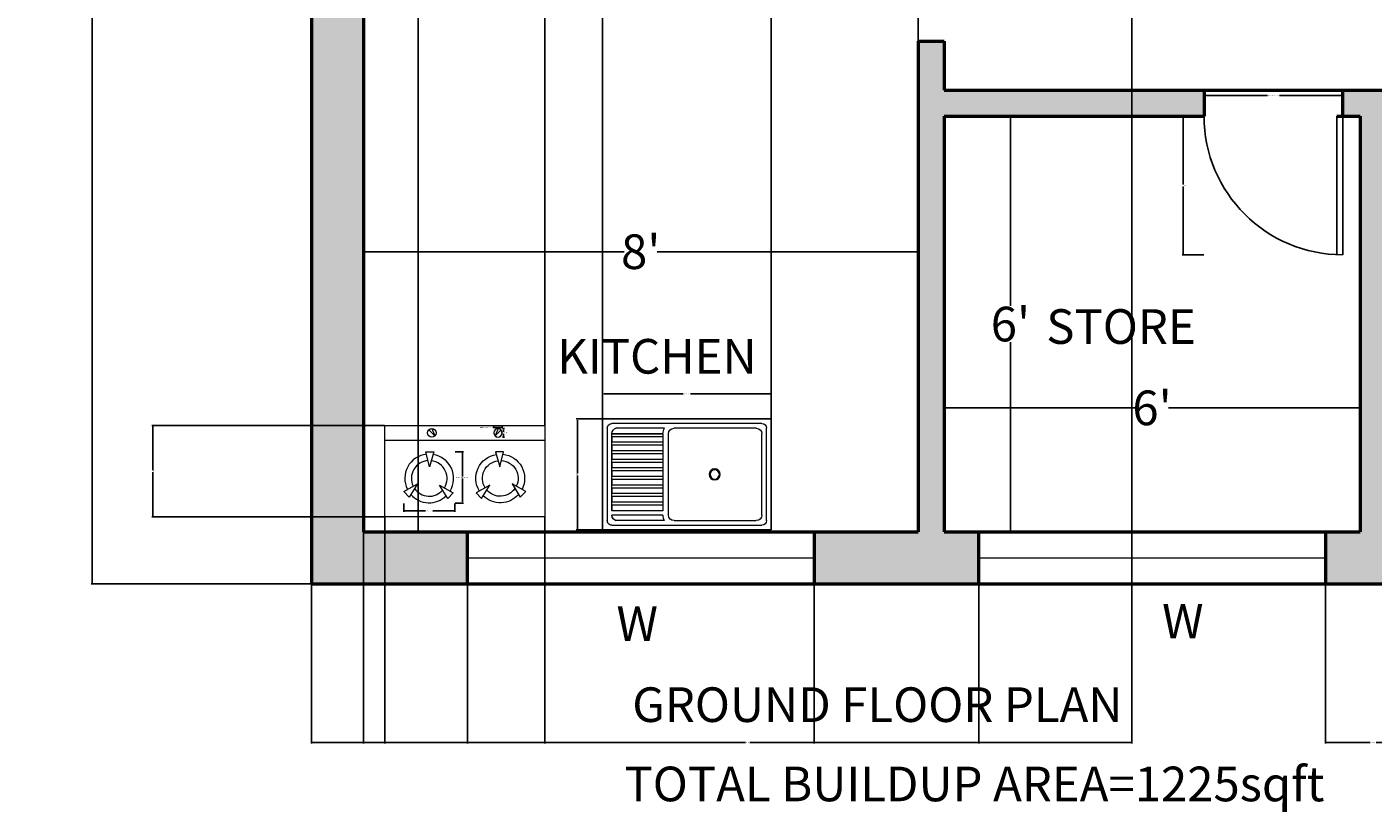
# Model space of a CAD drawing. Units: inches. Extents: x -22 to 470, y -437 to 97.
# Tile 1 of 9: x -22 to 211, y -437 to -301. Entities that reach past the tile are written whole.
import ezdxf

# ---------------------------------------------------------------- set-up
doc = ezdxf.new("R2010")
doc.units = ezdxf.units.IN
doc.header["$MEASUREMENT"] = 0
for name, color, linetype, lineweight in [('A-ANNO-DIMS', 2, 'Continuous', 18), ('A-ANNO-TEXT', 7, 'Continuous', 18), ('A-AREA-IDEN', 7, 'Continuous', 25), ('A-DOOR', 4, 'Continuous', 25), ('A-EQPM', 9, 'Continuous', 18), ('A-FLOR-FIXT', 9, 'Continuous', 20), ('A-GLAZ', 4, 'Continuous', 18), ('A-WALL', 7, 'Continuous', 50), ('A-WALL-PATT', 8, 'Continuous', 13)]:
    doc.layers.add(name, color=color, linetype=linetype, lineweight=lineweight)
doc.styles.get("Standard").update_dxf_attribs({"font": 'arial.ttf'})
doc.dimstyles.get("Standard").update_dxf_attribs({"dimtxt": 0.18, "dimasz": 0.18, "dimexe": 0.18, "dimexo": 0.0625, "dimgap": 0.09, "dimtad": 0, "dimtih": 1, "dimtoh": 1, "dimdec": 0, "dimzin": 0, "dimdsep": 46, "dimlunit": 3, "dimtxsty": 'Standard', "dimcen": 0.09, "dimadec": 0, "dimazin": 0, "dimtfac": 1, "dimtdec": 0, "dimtofl": 0, "dimtmove": 0, "dimatfit": 3, "dimfxl": 1, "dimtolj": 1, "dimtzin": 0, "dimarcsym": 0})

# ---------------------------------------------------------------- blocks, each defined once
blk = doc.blocks.new('М12 540х820')
for p, q in [((0, 540), (-820, 540)), ((-820, 540), (-820, 0)), ((0, 0), (0, 540)), ((-797.5, 495), (-797.5, 45)), ((-45, 517.5), (-775, 517.5)), ((-775, 468), (-775, 72)), ((-347.5, 495), (-748, 495)), ((-320.5, 468), (-320.5, 72)), ((-301.7, 495), (-64.8, 495)), ((-293.7, 468), (-293.7, 472.5)), ((-293.7, 468), (-45, 468)), ((-45, 469.5), (-45, 468)), ((-22.5, 45), (-22.5, 495)), ((-293.7, 446.6), (-45, 446.6)), ((-293.7, 419.6), (-293.7, 446.6)), ((-293.7, 419.6), (-45, 419.6)), ((-293.7, 405), (-45, 405)), ((-293.7, 378), (-293.7, 405)), ((-45, 419.6), (-45, 446.6)), ((-45, 378), (-45, 405)), ((-293.7, 378), (-45, 378)), ((-293.7, 336.4), (-293.7, 363.4)), ((-293.7, 363.4), (-45, 363.4)), ((-293.7, 336.4), (-45, 336.4)), ((-45, 336.4), (-45, 363.4)), ((-293.7, 294.7), (-293.7, 321.7)), ((-293.7, 321.7), (-45, 321.7)), ((-293.7, 294.7), (-45, 294.7)), ((-293.7, 253.1), (-293.7, 280.1)), ((-293.7, 280.1), (-45, 280.1)), ((-45, 294.7), (-45, 321.7)), ((-45, 253.1), (-45, 280.1)), ((-293.7, 253.1), (-45, 253.1)), ((-293.7, 211.5), (-293.7, 238.5)), ((-293.7, 238.5), (-45, 238.5)), ((-293.7, 211.5), (-45, 211.5)), ((-293.7, 169.9), (-293.7, 196.9)), ((-293.7, 196.9), (-45, 196.9)), ((-45, 211.5), (-45, 238.5)), ((-45, 169.9), (-45, 196.9)), ((-293.7, 169.9), (-45, 169.9)), ((-293.7, 128.2), (-293.7, 155.2)), ((-293.7, 155.2), (-45, 155.2)), ((-45, 128.2), (-45, 155.2)), ((-293.7, 128.2), (-45, 128.2)), ((-293.7, 113.6), (-45, 113.6)), ((-293.7, 86.6), (-293.7, 113.6)), ((-293.7, 86.6), (-45, 86.6)), ((-293.7, 72), (-45, 72)), ((-45, 86.6), (-45, 113.6)), ((-45, 70.5), (-45, 72)), ((-820, 0), (0, 0)), ((-775, 22.5), (-45, 22.5)), ((-748, 45), (-347.5, 45)), ((-301.7, 45), (-64.8, 45))]:
    blk.add_line(p, q)
at = {"ltscale": 0.06}
for p, q in [((-820, 0), (-820, 540)), ((-820, 540), (0, 540)), ((0, 540), (0, 536.9)), ((0, 536.9), (0, 0)), ((-293.7, 446.6), (-45, 446.6)), ((-293.7, 405), (-293.7, 446.6)), ((-293.7, 363.4), (-293.7, 405)), ((-45, 446.6), (-45, 419.6)), ((-45, 419.6), (-45, 378)), ((-293.7, 321.7), (-293.7, 363.4)), ((-45, 378), (-45, 336.4)), ((-45, 336.4), (-45, 294.7)), ((-293.7, 280.1), (-293.7, 321.7)), ((-293.7, 238.5), (-293.7, 280.1)), ((-45, 294.7), (-45, 253.1)), ((-293.7, 196.9), (-293.7, 238.5)), ((-293.7, 155.2), (-293.7, 196.9)), ((-45, 253.1), (-45, 211.5)), ((-45, 211.5), (-45, 169.9)), ((-293.7, 113.6), (-293.7, 155.2)), ((-45, 169.9), (-45, 128.2)), ((-293.7, 72), (-293.7, 113.6)), ((-45, 72), (-293.7, 72)), ((-45, 128.2), (-45, 86.6)), ((-45, 86.6), (-45, 72)), ((0, 0), (-820, 0))]:
    blk.add_line(p, q, dxfattribs=at)
at = {"extrusion": (0, 0, -1)}
for centre, major_axis, start_param, end_param in [((-775, 495), (-15.9, 15.9), -0.785398, 0.785398), ((-775, 495), (-15.9, 15.9), -0.785398, 0.785398), ((-748, 468), (-19.1, -19.1), 0.785398, 2.356194), ((-748, 468), (-19.1, -19.1), 0.785398, 2.356194), ((-347.5, 468), (-19.1, 19.1), 0.785398, 2.356194), ((-347.5, 468), (-19.1, 19.1), 0.785398, 2.356194), ((-343.2, 468), (-35, 35), 1.779263, 2.356194), ((-343.2, 468), (-35, 35), 1.779263, 2.356192), ((-343.2, 468), (-35, 35), 2.356192, 2.356194), ((-72.3, 468.8), (-19.3, 19.3), 1.0328, 2.38382), ((-72.3, 468.8), (-19.3, 19.3), 1.0328, 1.064673), ((-72.3, 468.8), (-19.3, 19.3), 1.064673, 2.328569), ((-45, 495), (-15.9, -15.9), 2.356194, 3.926991), ((-45, 495), (-15.9, -15.9), 2.356194, 3.926991), ((-72.3, 468.8), (-19.3, 19.3), 2.328569, 2.38382), ((-545.5, 270), (-19.1, -19.1), 3.926991, 10.210176), ((-545.5, 270), (-19.1, -19.1), 3.926991, 10.210176), ((-545.5, 270), (-15.9, -15.9), 3.926991, 10.210176), ((-545.5, 270), (-15.9, -15.9), 3.926991, 10.210176), ((-748, 72), (-19.1, 19.1), 3.926991, 5.497787), ((-748, 72), (-19.1, 19.1), 3.926991, 5.497787), ((-347.5, 72), (-19.1, -19.1), 3.926991, 5.497787), ((-347.5, 72), (-19.1, -19.1), 3.926991, 5.497787), ((-343.2, 72), (-35, -35), 3.926991, 4.503922), ((-343.2, 72), (-35, -35), 3.926991, 4.503922), ((-72.3, 71.2), (-19.3, -19.3), 3.899365, 5.250385), ((-72.3, 71.2), (-19.3, -19.3), 3.954617, 5.218512), ((-72.3, 71.2), (-19.3, -19.3), 3.899365, 3.954617), ((-775, 45), (-15.9, -15.9), 5.497787, 7.068583), ((-775, 45), (-15.9, -15.9), 5.497787, 7.068583), ((-72.3, 71.2), (-19.3, -19.3), 5.218512, 5.250385), ((-45, 45), (-15.9, 15.9), 2.356194, 3.926991), ((-45, 45), (-15.9, 15.9), 2.356194, 3.926991)]:
    blk.add_ellipse(centre, major_axis=major_axis, ratio=1, start_param=start_param, end_param=end_param, dxfattribs=at)
blk = doc.blocks.new('*D3')
at = {"layer": 'A-ANNO-DIMS', "color": 0, "lineweight": -2, "transparency": 16777216}
for p, q in [((26.86, 13.24), (-11.18, 13.24)), ((-11, 13.06), (-11, -189.1)), ((-11, -397.58), (-11, -195.41)), ((26.86, -397.76), (-11.18, -397.76))]:
    blk.add_line(p, q, dxfattribs=at)
at = {"layer": 'A-ANNO-DIMS', "color": 0, "transparency": 16777216}
for points in [[(-11.03, 13.06), (-10.97, 13.06), (-11, 13.24)], [(-11.03, -397.58), (-10.97, -397.58), (-11, -397.76)]]:
    blk.add_solid(points, dxfattribs=at)
at = {"layer": 'Defpoints', "color": 0, "transparency": 16777216}
for p in [(26.92, 13.24), (-11, -397.76), (26.92, -397.76)]:
    blk.add_point(p, dxfattribs=at)
at = {"layer": 'A-ANNO-DIMS', "color": 0, "transparency": 16777216, "insert": (-11, -192.26), "char_height": 6, "attachment_point": 5}
blk.add_mtext('\\A1;34\'-3"', dxfattribs=at)
blk = doc.blocks.new('*D15')
at = {"layer": 'A-ANNO-DIMS', "color": 0, "lineweight": -2, "transparency": 16777216}
for p, q in [((35.92, -346.19), (35.92, -340.05)), ((131.92, -346.19), (131.92, -340.05)), ((36.1, -340.23), (81.07, -340.23)), ((131.74, -340.23), (86.78, -340.23))]:
    blk.add_line(p, q, dxfattribs=at)
at = {"layer": 'A-ANNO-DIMS', "color": 0, "transparency": 16777216}
for points in [[(36.1, -340.2), (36.1, -340.26), (35.92, -340.23)], [(131.74, -340.2), (131.74, -340.26), (131.92, -340.23)]]:
    blk.add_solid(points, dxfattribs=at)
at = {"layer": 'Defpoints', "color": 0, "transparency": 16777216}
for p in [(35.92, -340.23), (35.92, -346.25), (131.92, -346.25)]:
    blk.add_point(p, dxfattribs=at)
at = {"layer": 'A-ANNO-DIMS', "color": 0, "transparency": 16777216, "insert": (83.92, -340.23), "char_height": 6, "attachment_point": 5}
blk.add_mtext("\\A1;8'", dxfattribs=at)
blk = doc.blocks.new('*D16')
at = {"layer": 'A-ANNO-DIMS', "color": 0, "lineweight": -2, "transparency": 16777216}
for p, q in [((136.42, -367.21), (136.42, -367.09)), ((136.6, -367.27), (169.55, -367.27)), ((208.24, -367.27), (175.29, -367.27)), ((208.42, -367.21), (208.42, -367.09))]:
    blk.add_line(p, q, dxfattribs=at)
at = {"layer": 'A-ANNO-DIMS', "color": 0, "transparency": 16777216}
for points in [[(136.6, -367.24), (136.6, -367.3), (136.42, -367.27)], [(208.24, -367.24), (208.24, -367.3), (208.42, -367.27)]]:
    blk.add_solid(points, dxfattribs=at)
at = {"layer": 'Defpoints', "color": 0, "transparency": 16777216}
for p in [(136.42, -367.27), (136.42, -367.27), (208.42, -367.27)]:
    blk.add_point(p, dxfattribs=at)
at = {"layer": 'A-ANNO-DIMS', "color": 0, "transparency": 16777216, "insert": (172.42, -367.27), "char_height": 6, "attachment_point": 5}
blk.add_mtext("\\A1;6'", dxfattribs=at)
blk = doc.blocks.new('*D17')
at = {"layer": 'A-ANNO-DIMS', "color": 0, "lineweight": -2, "transparency": 16777216}
for p, q in [((148.79, -316.76), (147.73, -316.76)), ((147.91, -316.94), (147.91, -349.6)), ((147.91, -388.58), (147.91, -355.91)), ((148.79, -388.76), (147.73, -388.76))]:
    blk.add_line(p, q, dxfattribs=at)
at = {"layer": 'A-ANNO-DIMS', "color": 0, "transparency": 16777216}
for points in [[(147.88, -316.94), (147.94, -316.94), (147.91, -316.76)], [(147.88, -388.58), (147.94, -388.58), (147.91, -388.76)]]:
    blk.add_solid(points, dxfattribs=at)
at = {"layer": 'Defpoints', "color": 0, "transparency": 16777216}
for p in [(148.85, -316.76), (147.91, -388.76), (148.85, -388.76)]:
    blk.add_point(p, dxfattribs=at)
at = {"layer": 'A-ANNO-DIMS', "color": 0, "transparency": 16777216, "insert": (147.91, -352.76), "char_height": 6, "attachment_point": 5}
blk.add_mtext("\\A1;6'", dxfattribs=at)
blk = doc.blocks.new('*D20')
at = {"layer": 'A-ANNO-DIMS', "color": 0, "lineweight": -2, "transparency": 16777216}
for p, q in [((45.66, -196.76), (45.23, -196.76)), ((45.41, -196.94), (45.41, -289.6)), ((45.41, -388.58), (45.41, -295.91)), ((45.66, -388.76), (45.23, -388.76))]:
    blk.add_line(p, q, dxfattribs=at)
at = {"layer": 'A-ANNO-DIMS', "color": 0, "transparency": 16777216}
for points in [[(45.38, -196.94), (45.44, -196.94), (45.41, -196.76)], [(45.38, -388.58), (45.44, -388.58), (45.41, -388.76)]]:
    blk.add_solid(points, dxfattribs=at)
at = {"layer": 'Defpoints', "color": 0, "transparency": 16777216}
for p in [(45.73, -196.76), (45.41, -388.76), (45.73, -388.76)]:
    blk.add_point(p, dxfattribs=at)
at = {"layer": 'A-ANNO-DIMS', "color": 0, "transparency": 16777216, "insert": (45.41, -292.76), "char_height": 6, "attachment_point": 5}
blk.add_mtext("\\A1;16'", dxfattribs=at)
blk = doc.blocks.new('DOOR-SWING-24')
for p, q in [((23, 24), (23, 0)), ((24, 24), (24, 0))]:
    blk.add_line(p, q)
blk.add_arc((24, 24), 24, 180, 270)
blk = doc.blocks.new('COOKTOP-BURNER')
for p, q in [((4.49, 6.22), (3.84, 8.82)), ((3.84, 8.82), (5.21, 8.82)), ((5.21, 8.82), (4.49, 6.22)), ((0, 1.96), (2.36, 3.28)), ((2.36, 3.28), (0.96, 0.99)), ((7.64, 0.74), (6.21, 3.03)), ((6.21, 3.03), (8.57, 1.74)), ((0.96, 0.99), (0, 1.96)), ((8.57, 1.74), (7.64, 0.74))]:
    blk.add_line(p, q)
for radius, start, end in [(4.22, 96.4005, 206.769), (3.09, 93.5753, 205.9207), (3.09, 327.9778, 83.02), (4.22, 328.853, 80.7562), (3.09, 214.5561, 318.8027), (4.22, 221.2225, 314.1627)]:
    blk.add_arc((4.41, 4.22), radius, start, end)
blk = doc.blocks.new('COOKTOP-DIAL')
at = {"ltscale": 20}
for p, q in [((1.25, 0.22), (0.21, 1.24)), ((0.73, 1.46), (1.25, 0.22))]:
    blk.add_line(p, q, dxfattribs=at)
blk.add_circle((0.73, 0.73), 0.728, dxfattribs=at)
blk = doc.blocks.new('WINDOW-60-SASH')
for p, q in [((0, 9), (60, 9)), ((0, 4.5), (60, 4.5)), ((60, 0), (0, 0))]:
    blk.add_line(p, q)
blk = doc.blocks.new('*D37')
at = {"layer": 'A-ANNO-DIMS', "color": 0, "lineweight": -2, "transparency": 16777216}
for p, q in [((181.42, -316.69), (181.42, -312.98)), ((181.6, -313.16), (192.38, -313.16)), ((205.24, -313.16), (194.47, -313.16)), ((205.42, -316.69), (205.42, -312.98))]:
    blk.add_line(p, q, dxfattribs=at)
at = {"layer": 'A-ANNO-DIMS', "color": 0, "transparency": 16777216}
for points in [[(181.6, -313.13), (181.6, -313.19), (181.42, -313.16)], [(205.24, -313.13), (205.24, -313.19), (205.42, -313.16)]]:
    blk.add_solid(points, dxfattribs=at)
at = {"layer": 'Defpoints', "color": 0, "transparency": 16777216}
for p in [(205.42, -313.16), (181.42, -316.76), (205.42, -316.76)]:
    blk.add_point(p, dxfattribs=at)
at = {"layer": 'A-ANNO-DIMS', "color": 0, "transparency": 16777216, "insert": (193.42, -313.16), "char_height": 0.18, "attachment_point": 5}
blk.add_mtext('\\A1;DOOR 2\'-0" TYP.', dxfattribs=at)
blk = doc.blocks.new('*D38')
at = {"layer": 'A-ANNO-DIMS', "color": 0, "lineweight": -2, "transparency": 16777216}
for p, q in [((181.36, -316.76), (177.64, -316.76)), ((177.82, -316.94), (177.82, -328.57)), ((177.82, -340.58), (177.82, -328.94)), ((181.36, -340.76), (177.64, -340.76))]:
    blk.add_line(p, q, dxfattribs=at)
at = {"layer": 'A-ANNO-DIMS', "color": 0, "transparency": 16777216}
for points in [[(177.79, -316.94), (177.85, -316.94), (177.82, -316.76)], [(177.79, -340.58), (177.85, -340.58), (177.82, -340.76)]]:
    blk.add_solid(points, dxfattribs=at)
at = {"layer": 'Defpoints', "color": 0, "transparency": 16777216}
for p in [(177.82, -316.76), (181.42, -316.76), (181.42, -340.76)]:
    blk.add_point(p, dxfattribs=at)
at = {"layer": 'A-ANNO-DIMS', "color": 0, "transparency": 16777216, "insert": (177.82, -328.76), "char_height": 0.18, "attachment_point": 5}
blk.add_mtext('\\A1;2\'-0" TYP.', dxfattribs=at)
blk = doc.blocks.new('*D55')
at = {"layer": 'A-ANNO-DIMS', "color": 0, "lineweight": -2, "transparency": 16777216}
for p, q in [((58.49, -370.65), (58.31, -370.65)), ((58.49, -370.81), (58.49, -370.47)), ((59.77, -370.65), (58.67, -370.65)), ((59.95, -370.81), (59.95, -370.47))]:
    blk.add_line(p, q, dxfattribs=at)
at = {"layer": 'A-ANNO-DIMS', "color": 0, "transparency": 16777216}
for points in [[(58.67, -370.62), (58.67, -370.68), (58.49, -370.65)], [(59.77, -370.62), (59.77, -370.68), (59.95, -370.65)]]:
    blk.add_solid(points, dxfattribs=at)
at = {"layer": 'Defpoints', "color": 0, "transparency": 16777216}
for p in [(58.49, -370.65), (58.49, -370.87), (59.95, -370.87)]:
    blk.add_point(p, dxfattribs=at)
at = {"layer": 'A-ANNO-DIMS', "color": 0, "transparency": 16777216, "insert": (57.15, -370.65), "char_height": 0.18, "attachment_point": 5}
blk.add_mtext('\\A1;DIAL 0\'-1 1/2" TYP.', dxfattribs=at)
blk = doc.blocks.new('*D56')
at = {"layer": 'A-ANNO-DIMS', "color": 0, "lineweight": -2, "transparency": 16777216}
for p, q in [((60.01, -370.87), (60.35, -370.87)), ((60.01, -372.33), (60.35, -372.33)), ((60.17, -371.05), (60.17, -371.42)), ((60.17, -372.15), (60.17, -371.78))]:
    blk.add_line(p, q, dxfattribs=at)
at = {"layer": 'A-ANNO-DIMS', "color": 0, "transparency": 16777216}
for points in [[(60.14, -371.05), (60.2, -371.05), (60.17, -370.87)], [(60.14, -372.15), (60.2, -372.15), (60.17, -372.33)]]:
    blk.add_solid(points, dxfattribs=at)
at = {"layer": 'Defpoints', "color": 0, "transparency": 16777216}
for p in [(59.95, -370.87), (59.95, -372.33), (60.17, -370.87)]:
    blk.add_point(p, dxfattribs=at)
at = {"layer": 'A-ANNO-DIMS', "color": 0, "transparency": 16777216, "insert": (60.17, -371.6), "char_height": 0.18, "attachment_point": 5}
blk.add_mtext('\\A1;0\'-1 1/2" TYP.', dxfattribs=at)
blk = doc.blocks.new('*D57')
at = {"layer": 'A-ANNO-DIMS', "color": 0, "lineweight": -2, "transparency": 16777216}
for p, q in [((51.8, -374.88), (53.24, -374.88)), ((53.06, -375.06), (53.06, -379.13)), ((53.06, -383.57), (53.06, -379.5)), ((51.8, -383.75), (53.24, -383.75))]:
    blk.add_line(p, q, dxfattribs=at)
at = {"layer": 'A-ANNO-DIMS', "color": 0, "transparency": 16777216}
for points in [[(53.03, -375.06), (53.09, -375.06), (53.06, -374.88)], [(53.03, -383.57), (53.09, -383.57), (53.06, -383.75)]]:
    blk.add_solid(points, dxfattribs=at)
at = {"layer": 'Defpoints', "color": 0, "transparency": 16777216}
for p in [(51.73, -374.88), (53.06, -374.88), (51.73, -383.75)]:
    blk.add_point(p, dxfattribs=at)
at = {"layer": 'A-ANNO-DIMS', "color": 0, "transparency": 16777216, "insert": (53.06, -379.32), "char_height": 0.18, "attachment_point": 5}
blk.add_mtext('\\A1;BURNER 0\'-9" TYP.', dxfattribs=at)
blk = doc.blocks.new('*D58')
at = {"layer": 'A-ANNO-DIMS', "color": 0, "lineweight": -2, "transparency": 16777216}
for p, q in [((42.9, -383.81), (42.9, -385.26)), ((51.73, -383.81), (51.73, -385.26)), ((43.08, -385.08), (46.68, -385.08)), ((51.55, -385.08), (47.96, -385.08))]:
    blk.add_line(p, q, dxfattribs=at)
at = {"layer": 'A-ANNO-DIMS', "color": 0, "transparency": 16777216}
for points in [[(43.08, -385.05), (43.08, -385.11), (42.9, -385.08)], [(51.55, -385.05), (51.55, -385.11), (51.73, -385.08)]]:
    blk.add_solid(points, dxfattribs=at)
at = {"layer": 'Defpoints', "color": 0, "transparency": 16777216}
for p in [(42.9, -383.75), (51.73, -383.75), (51.73, -385.08)]:
    blk.add_point(p, dxfattribs=at)
at = {"layer": 'A-ANNO-DIMS', "color": 0, "transparency": 16777216, "insert": (47.32, -385.08), "char_height": 0.18, "attachment_point": 5}
blk.add_mtext('\\A1;0\'-9" TYP.', dxfattribs=at)
blk = doc.blocks.new('*D59')
at = {"layer": 'A-ANNO-DIMS', "color": 0, "lineweight": -2, "transparency": 16777216}
for p, q in [((77.33, -369.14), (77.33, -364.65)), ((77.51, -364.83), (91.25, -364.83)), ((106.3, -364.83), (92.56, -364.83)), ((106.48, -369.14), (106.48, -364.65))]:
    blk.add_line(p, q, dxfattribs=at)
at = {"layer": 'A-ANNO-DIMS', "color": 0, "transparency": 16777216}
for points in [[(77.51, -364.8), (77.51, -364.86), (77.33, -364.83)], [(106.3, -364.8), (106.3, -364.86), (106.48, -364.83)]]:
    blk.add_solid(points, dxfattribs=at)
at = {"layer": 'Defpoints', "color": 0, "transparency": 16777216}
for p in [(77.33, -364.83), (77.33, -369.2), (106.48, -369.2)]:
    blk.add_point(p, dxfattribs=at)
at = {"layer": 'A-ANNO-DIMS', "color": 0, "transparency": 16777216, "insert": (91.91, -364.83), "char_height": 0.18, "attachment_point": 5}
blk.add_mtext('\\A1;SINK 2\'-5"', dxfattribs=at)
blk = doc.blocks.new('*D60')
at = {"layer": 'A-ANNO-DIMS', "color": 0, "lineweight": -2, "transparency": 16777216}
for p, q in [((77.27, -369.2), (72.77, -369.2)), ((72.95, -369.38), (72.95, -378.62)), ((72.95, -388.22), (72.95, -378.98)), ((77.27, -388.4), (72.77, -388.4))]:
    blk.add_line(p, q, dxfattribs=at)
at = {"layer": 'A-ANNO-DIMS', "color": 0, "transparency": 16777216}
for points in [[(72.92, -369.38), (72.98, -369.38), (72.95, -369.2)], [(72.92, -388.22), (72.98, -388.22), (72.95, -388.4)]]:
    blk.add_solid(points, dxfattribs=at)
at = {"layer": 'Defpoints', "color": 0, "transparency": 16777216}
for p in [(77.33, -369.2), (72.95, -388.4), (77.33, -388.4)]:
    blk.add_point(p, dxfattribs=at)
at = {"layer": 'A-ANNO-DIMS', "color": 0, "transparency": 16777216, "insert": (72.95, -378.8), "char_height": 0.18, "attachment_point": 5}
blk.add_mtext('\\A1;1\'-7"', dxfattribs=at)
blk = doc.blocks.new('*D62')
at = {"layer": 'A-ANNO-DIMS', "color": 0, "lineweight": -2, "transparency": 16777216}
for p, q in [((35.92, -192.32), (35.92, -425.39)), ((168.92, -192.32), (168.92, -425.39)), ((36.1, -425.21), (102.03, -425.21)), ((168.74, -425.21), (102.81, -425.21))]:
    blk.add_line(p, q, dxfattribs=at)
at = {"layer": 'A-ANNO-DIMS', "color": 0, "transparency": 16777216}
for points in [[(36.1, -425.18), (36.1, -425.24), (35.92, -425.21)], [(168.74, -425.18), (168.74, -425.24), (168.92, -425.21)]]:
    blk.add_solid(points, dxfattribs=at)
at = {"layer": 'Defpoints', "color": 0, "transparency": 16777216}
for p in [(35.92, -192.26), (168.92, -192.26), (168.92, -425.21)]:
    blk.add_point(p, dxfattribs=at)
at = {"layer": 'A-ANNO-DIMS', "color": 0, "transparency": 16777216, "insert": (102.42, -425.21), "char_height": 0.18, "attachment_point": 5}
blk.add_mtext('\\A1;11\'-1"', dxfattribs=at)
blk = doc.blocks.new('*D72')
at = {"layer": 'A-ANNO-DIMS', "color": 0, "lineweight": -2, "transparency": 16777216}
for p, q in [((26.92, -397.82), (26.92, -425.39)), ((53.92, -397.82), (53.92, -425.39)), ((27.1, -425.21), (40.09, -425.21)), ((53.74, -425.21), (40.75, -425.21))]:
    blk.add_line(p, q, dxfattribs=at)
at = {"layer": 'A-ANNO-DIMS', "color": 0, "transparency": 16777216}
for points in [[(27.1, -425.18), (27.1, -425.24), (26.92, -425.21)], [(53.74, -425.18), (53.74, -425.24), (53.92, -425.21)]]:
    blk.add_solid(points, dxfattribs=at)
at = {"layer": 'Defpoints', "color": 0, "transparency": 16777216}
for p in [(26.92, -397.76), (53.92, -397.76), (53.92, -425.21)]:
    blk.add_point(p, dxfattribs=at)
at = {"layer": 'A-ANNO-DIMS', "color": 0, "transparency": 16777216, "insert": (40.42, -425.21), "char_height": 0.18, "attachment_point": 5}
blk.add_mtext('\\A1;2\'-3"', dxfattribs=at)
blk = doc.blocks.new('*D73')
at = {"layer": 'A-ANNO-DIMS', "color": 0, "lineweight": -2, "transparency": 16777216}
for p, q in [((113.92, -397.82), (113.92, -425.39)), ((142.42, -397.82), (142.42, -425.39)), ((114.1, -425.21), (127.63, -425.21)), ((142.24, -425.21), (128.71, -425.21))]:
    blk.add_line(p, q, dxfattribs=at)
at = {"layer": 'A-ANNO-DIMS', "color": 0, "transparency": 16777216}
for points in [[(114.1, -425.18), (114.1, -425.24), (113.92, -425.21)], [(142.24, -425.18), (142.24, -425.24), (142.42, -425.21)]]:
    blk.add_solid(points, dxfattribs=at)
at = {"layer": 'Defpoints', "color": 0, "transparency": 16777216}
for p in [(113.92, -397.76), (142.42, -397.76), (142.42, -425.21)]:
    blk.add_point(p, dxfattribs=at)
at = {"layer": 'A-ANNO-DIMS', "color": 0, "transparency": 16777216, "insert": (128.17, -425.21), "char_height": 0.18, "attachment_point": 5}
blk.add_mtext('\\A1;2\'-4 1/2"', dxfattribs=at)
blk = doc.blocks.new('*D74')
at = {"layer": 'A-ANNO-DIMS', "color": 0, "lineweight": -2, "transparency": 16777216}
for p, q in [((202.42, -397.82), (202.42, -425.39)), ((218.92, -397.82), (218.92, -425.39)), ((202.6, -425.21), (210.14, -425.21)), ((218.74, -425.21), (211.2, -425.21))]:
    blk.add_line(p, q, dxfattribs=at)
at = {"layer": 'A-ANNO-DIMS', "color": 0, "transparency": 16777216}
for points in [[(202.6, -425.18), (202.6, -425.24), (202.42, -425.21)], [(218.74, -425.18), (218.74, -425.24), (218.92, -425.21)]]:
    blk.add_solid(points, dxfattribs=at)
at = {"layer": 'Defpoints', "color": 0, "transparency": 16777216}
for p in [(202.42, -397.76), (218.92, -397.76), (218.92, -425.21)]:
    blk.add_point(p, dxfattribs=at)
at = {"layer": 'A-ANNO-DIMS', "color": 0, "transparency": 16777216, "insert": (210.67, -425.21), "char_height": 0.18, "attachment_point": 5}
blk.add_mtext('\\A1;1\'-4 1/2"', dxfattribs=at)
blk = doc.blocks.new('*D81')
at = {"layer": 'A-ANNO-DIMS', "color": 0, "lineweight": -2, "transparency": 16777216}
for p, q in [((39.64, -386.21), (39.64, -425.39)), ((67.35, -386.21), (67.35, -425.39)), ((39.82, -425.21), (52.95, -425.21)), ((67.17, -425.21), (54.04, -425.21))]:
    blk.add_line(p, q, dxfattribs=at)
at = {"layer": 'A-ANNO-DIMS', "color": 0, "transparency": 16777216}
for points in [[(39.82, -425.18), (39.82, -425.24), (39.64, -425.21)], [(67.17, -425.18), (67.17, -425.24), (67.35, -425.21)]]:
    blk.add_solid(points, dxfattribs=at)
at = {"layer": 'Defpoints', "color": 0, "transparency": 16777216}
for p in [(39.64, -386.15), (67.35, -386.15), (67.35, -425.21)]:
    blk.add_point(p, dxfattribs=at)
at = {"layer": 'A-ANNO-DIMS', "color": 0, "transparency": 16777216, "insert": (53.49, -425.21), "char_height": 0.18, "attachment_point": 5}
blk.add_mtext('\\A1;2\'-3 1/2"', dxfattribs=at)
blk = doc.blocks.new('*D82')
at = {"layer": 'A-ANNO-DIMS', "color": 0, "lineweight": -2, "transparency": 16777216}
for p, q in [((39.58, -370.32), (-0.71, -370.32)), ((-0.53, -370.5), (-0.53, -378.05)), ((-0.53, -385.97), (-0.53, -378.41)), ((39.58, -386.15), (-0.71, -386.15))]:
    blk.add_line(p, q, dxfattribs=at)
at = {"layer": 'A-ANNO-DIMS', "color": 0, "transparency": 16777216}
for points in [[(-0.56, -370.5), (-0.5, -370.5), (-0.53, -370.32)], [(-0.56, -385.97), (-0.5, -385.97), (-0.53, -386.15)]]:
    blk.add_solid(points, dxfattribs=at)
at = {"layer": 'Defpoints', "color": 0, "transparency": 16777216}
for p in [(39.64, -370.32), (-0.53, -386.15), (39.64, -386.15)]:
    blk.add_point(p, dxfattribs=at)
at = {"layer": 'A-ANNO-DIMS', "color": 0, "transparency": 16777216, "insert": (-0.53, -378.23), "char_height": 0.18, "attachment_point": 5}
blk.add_mtext('\\A1;1\'-4"', dxfattribs=at)
blk = doc.blocks.new('*D83')
at = {"layer": 'A-ANNO-DIMS', "color": 0, "lineweight": -2, "transparency": 16777216}
for p, q in [((67.35, -370.26), (67.35, 40.87)), ((67.53, 40.69), (71.94, 40.69)), ((77.15, 40.69), (72.74, 40.69)), ((77.33, -369.14), (77.33, 40.87))]:
    blk.add_line(p, q, dxfattribs=at)
at = {"layer": 'A-ANNO-DIMS', "color": 0, "transparency": 16777216}
for points in [[(67.53, 40.72), (67.53, 40.66), (67.35, 40.69)], [(77.15, 40.72), (77.15, 40.66), (77.33, 40.69)]]:
    blk.add_solid(points, dxfattribs=at)
at = {"layer": 'Defpoints', "color": 0, "transparency": 16777216}
for p in [(77.33, 40.69), (67.35, -370.32), (77.33, -369.2)]:
    blk.add_point(p, dxfattribs=at)
at = {"layer": 'A-ANNO-DIMS', "color": 0, "transparency": 16777216, "insert": (72.34, 40.69), "char_height": 0.18, "attachment_point": 5}
blk.add_mtext('\\A1;0\'-10"', dxfattribs=at)
blk = doc.blocks.new('*D84')
at = {"layer": 'A-ANNO-DIMS', "color": 0, "lineweight": -2, "transparency": 16777216}
for p, q in [((106.48, -369.14), (106.48, 40.87)), ((106.66, 40.69), (118.66, 40.69)), ((131.74, 40.69), (119.74, 40.69)), ((131.92, -388.69), (131.92, 40.87))]:
    blk.add_line(p, q, dxfattribs=at)
at = {"layer": 'A-ANNO-DIMS', "color": 0, "transparency": 16777216}
for points in [[(106.66, 40.72), (106.66, 40.66), (106.48, 40.69)], [(131.74, 40.72), (131.74, 40.66), (131.92, 40.69)]]:
    blk.add_solid(points, dxfattribs=at)
at = {"layer": 'Defpoints', "color": 0, "transparency": 16777216}
for p in [(131.92, 40.69), (106.48, -369.2), (131.92, -388.76)]:
    blk.add_point(p, dxfattribs=at)
at = {"layer": 'A-ANNO-DIMS', "color": 0, "transparency": 16777216, "insert": (119.2, 40.69), "char_height": 0.18, "attachment_point": 5}
blk.add_mtext('\\A1;2\'-1 1/2"', dxfattribs=at)

msp = doc.modelspace()

# ---------------------------------------------------------------- hatches: boundary and pattern name
at = {"layer": 'A-WALL-PATT'}
h = msp.add_hatch(color=256, dxfattribs=at)
h.dxf.hatch_style = 1
h.paths.add_polyline_path([(130.42, 13.24), (26.92, 13.24), (26.92, -43.76), (35.92, -43.76), (35.92, 4.24), (83.92, 4.24), (83.92, 1.24), (88.42, 1.24), (88.42, 4.24), (130.42, 4.24)])
h.paths.add_polyline_path([(266.92, 13.24), (190.42, 13.24), (190.42, 4.24), (232.42, 4.24), (232.42, -115.76), (229.42, -115.76), (229.42, -120.26), (239.92, -120.26), (239.92, -115.76), (236.92, -115.76), (236.92, 4.24), (266.92, 4.24)])
h.paths.add_polyline_path([(442.42, 13.24), (326.92, 13.24), (326.92, 4.24), (356.92, 4.24), (356.92, 1.24), (361.42, 1.24), (361.42, 4.24), (433.42, 4.24), (433.42, -49.38), (442.42, -49.38)])
h.paths.add_polyline_path([(442.42, -73.38), (433.42, -73.38), (433.42, -115.76), (361.42, -115.76), (361.42, -22.76), (356.92, -22.76), (356.92, -115.76), (263.92, -115.76), (263.92, -120.26), (332.92, -120.26), (332.92, -123.26), (337.42, -123.26), (337.42, -120.26), (433.42, -120.26), (433.42, -148.49), (442.42, -148.49)])
h.paths.add_polyline_path([(205.42, -115.76), (88.42, -115.76), (88.42, -22.76), (83.92, -22.76), (83.92, -115.76), (35.92, -115.76), (35.92, -67.76), (26.92, -67.76), (26.92, -126.26), (35.92, -126.26), (35.92, -120.26), (205.42, -120.26)])
h.paths.add_polyline_path([(35.92, -196.76), (168.92, -196.76), (168.92, -192.26), (35.92, -192.26), (35.92, -186.26), (26.92, -186.26), (26.92, -224.25), (35.92, -224.25)])
h.paths.add_polyline_path([(35.92, -284.25), (26.92, -284.25), (26.92, -397.76), (53.92, -397.76), (53.92, -388.76), (35.92, -388.76)])
h.paths.add_polyline_path([(142.42, -388.76), (136.42, -388.76), (136.42, -316.76), (181.42, -316.76), (181.42, -312.26), (136.42, -312.26), (136.42, -303.75), (131.92, -303.75), (131.92, -388.76), (113.92, -388.76), (113.92, -397.76), (142.42, -397.76)])
h.paths.add_polyline_path([(218.92, -388.76), (212.92, -388.76), (212.92, -312.26), (205.42, -312.26), (205.42, -316.76), (208.42, -316.76), (208.42, -388.76), (202.42, -388.76), (202.42, -397.76), (218.92, -397.76)])
h.paths.add_polyline_path([(306.75, -388.76), (289.42, -388.76), (289.42, -316.76), (284.92, -316.76), (284.92, -388.76), (278.92, -388.76), (278.92, -397.76), (306.75, -397.76)])
h.paths.add_polyline_path([(391.42, -388.76), (366.75, -388.76), (366.75, -397.76), (391.42, -397.76)], flags=17)
h.paths.add_polyline_path([(442.42, -172.49), (433.42, -172.49), (433.42, -192.26), (337.42, -192.26), (337.42, -147.26), (332.92, -147.26), (332.92, -196.76), (433.42, -196.76), (433.42, -388.76), (427.42, -388.76), (427.42, -397.76), (442.42, -397.76)])

# ---------------------------------------------------------------- linework, layer by layer
at = {"layer": 'A-EQPM'}
msp.add_line((39.64, -372.89), (67.35, -372.89), dxfattribs=at)
msp.add_lwpolyline([(67.35, -386.15), (39.64, -386.15), (39.64, -370.32), (67.35, -370.32)], close=True, dxfattribs=at)
at = {"layer": 'A-WALL'}
for p, q in [((26.92, 13.24), (26.92, -397.76)), ((35.92, -196.76), (35.92, -388.76)), ((131.92, -303.75), (131.92, -388.76)), ((131.92, -303.75), (136.42, -303.75)), ((136.42, -303.75), (136.42, -312.26)), ((136.42, -312.26), (212.92, -312.26)), ((181.42, -312.26), (181.42, -316.76)), ((205.42, -316.76), (205.42, -312.26)), ((136.42, -316.76), (181.42, -316.76)), ((136.42, -316.76), (136.42, -388.76)), ((204.42, -316.76), (208.42, -316.76)), ((208.42, -316.76), (208.42, -388.76)), ((35.92, -388.76), (131.92, -388.76)), ((53.92, -397.76), (53.92, -388.76)), ((113.92, -388.76), (113.92, -397.76)), ((136.42, -388.76), (208.42, -388.76)), ((142.42, -397.76), (142.42, -388.76)), ((202.42, -388.76), (202.42, -397.76)), ((26.92, -397.76), (391.42, -397.76))]:
    msp.add_line(p, q, dxfattribs=at)

# ---------------------------------------------------------------- block references
at = {"layer": 'A-DOOR'}
msp.add_blockref('DOOR-SWING-24', (181.42, -340.76), dxfattribs=at)
at = {"layer": 'A-EQPM'}
for name, p in [('COOKTOP-DIAL', (47.04, -372.33)), ('COOKTOP-BURNER', (42.9, -383.71))]:
    msp.add_blockref(name, p, dxfattribs=at)
at = {"layer": 'A-EQPM', "extrusion": (0, 0, -1), "zscale": -1}
for name, p in [('COOKTOP-DIAL', (-59.95, -372.33)), ('COOKTOP-BURNER', (-64.02, -383.71))]:
    msp.add_blockref(name, p, dxfattribs=at)
at = {"layer": 'A-FLOR-FIXT', "xscale": 0.0355567693074003, "yscale": 0.0355567693074003, "zscale": 0.0355567693074003, "rotation": 180}
msp.add_blockref('М12 540х820', (77.33, -369.2), dxfattribs=at)
at = {"layer": 'A-GLAZ'}
for p in [(53.92, -397.76), (142.42, -397.76)]:
    msp.add_blockref('WINDOW-60-SASH', p, dxfattribs=at)

# ---------------------------------------------------------------- texts
at = {"layer": 'A-ANNO-TEXT', "char_height": 6, "attachment_point": 1}
for s, insert in [('W', (79.72, -401.63)), ('W', (174.15, -401.21)), ('GROUND FLOOR PLAN', (82.45, -415.67)), ('TOTAL BUILDUP AREA=1225sqft', (81.1, -429.4))]:
    msp.add_mtext(s, dxfattribs=dict(at, insert=insert))
at = {"layer": 'A-AREA-IDEN', "char_height": 6, "attachment_point": 1}
for s, insert in [('STORE', (154.11, -350.19)), ('KITCHEN', (69.48, -355.34))]:
    msp.add_mtext(s, dxfattribs=dict(at, insert=insert))

# ---------------------------------------------------------------- dimensions: what is measured, and where the dimension line sits
at = {"layer": 'A-ANNO-DIMS'}
for base, p1, p2, override, picture, middle in [((77.33, 40.69), (67.35, -370.32), (77.33, -369.2), {"dimdec": 1, "dimlfac": 1, "dimrnd": 0, "dimzin": 1, "dimdsep": 46, "dimlunit": 4, "dimfrac": 2}, '*D83', (72.34, 40.69)), ((131.92, 40.69), (106.48, -369.2), (131.92, -388.76), {"dimdec": 1, "dimlfac": 1, "dimrnd": 0, "dimzin": 1, "dimdsep": 46, "dimlunit": 4, "dimfrac": 2}, '*D84', (119.2, 40.69)), ((168.92, -425.21), (35.92, -192.26), (168.92, -192.26), {"dimdec": 1, "dimlfac": 1, "dimrnd": 0, "dimzin": 1, "dimdsep": 46, "dimlunit": 4, "dimfrac": 2}, '*D62', (102.42, -425.21)), ((35.92, -340.23), (131.92, -346.25), (35.92, -346.25), {"dimtxt": 6, "dimclrd": 0, "dimclre": 0, "dimclrt": 0}, '*D15', (83.92, -340.23)), ((136.42, -367.27), (208.42, -367.27), (136.42, -367.27), {"dimtxt": 6, "dimclrd": 0, "dimclre": 0, "dimclrt": 0}, '*D16', (172.42, -367.27)), ((67.35, -425.21), (39.64, -386.15), (67.35, -386.15), {"dimdec": 1, "dimlfac": 1, "dimrnd": 0, "dimzin": 1, "dimdsep": 46, "dimlunit": 4, "dimfrac": 2}, '*D81', (53.49, -425.21)), ((53.92, -425.21), (26.92, -397.76), (53.92, -397.76), {"dimdec": 1, "dimlfac": 1, "dimrnd": 0, "dimzin": 1, "dimdsep": 46, "dimlunit": 4, "dimfrac": 2}, '*D72', (40.42, -425.21)), ((142.42, -425.21), (113.92, -397.76), (142.42, -397.76), {"dimdec": 1, "dimlfac": 1, "dimrnd": 0, "dimzin": 1, "dimdsep": 46, "dimlunit": 4, "dimfrac": 2}, '*D73', (128.17, -425.21)), ((218.92, -425.21), (202.42, -397.76), (218.92, -397.76), {"dimdec": 1, "dimlfac": 1, "dimrnd": 0, "dimzin": 1, "dimdsep": 46, "dimlunit": 4, "dimfrac": 2}, '*D74', (210.67, -425.21))]:
    dim = msp.add_linear_dim(base=base, p1=p1, p2=p2, dimstyle='Standard', override=override, dxfattribs=at)
    dim.commit()
    dim.dimension.update_dxf_attribs({"geometry": picture, "text_midpoint": middle})
for base, p1, p2, angle, override, picture, middle in [((-11, -397.76), (26.92, 13.24), (26.92, -397.76), 90, {"dimtxt": 6, "dimclrd": 0, "dimclre": 0, "dimclrt": 0}, '*D3', (-11, -192.26)), ((45.41, -388.76), (45.73, -196.76), (45.73, -388.76), 90, {"dimtxt": 6, "dimclrd": 0, "dimclre": 0, "dimclrt": 0}, '*D20', (45.41, -292.76)), ((147.91, -388.76), (148.85, -316.76), (148.85, -388.76), 90, {"dimtxt": 6, "dimclrd": 0, "dimclre": 0, "dimclrt": 0}, '*D17', (147.91, -352.76)), ((-0.53, -386.15), (39.64, -370.32), (39.64, -386.15), 90, {"dimdec": 1, "dimlfac": 1, "dimrnd": 0, "dimzin": 1, "dimdsep": 46, "dimlunit": 4, "dimfrac": 2}, '*D82', (-0.53, -378.23)), ((72.95, -388.4), (77.33, -369.2), (77.33, -388.4), 270, {"dimdec": 1, "dimlfac": 1, "dimrnd": 0, "dimzin": 1, "dimdsep": 46, "dimlunit": 4, "dimfrac": 2}, '*D60', (72.95, -378.8))]:
    dim = msp.add_linear_dim(base=base, p1=p1, p2=p2, angle=angle, dimstyle='Standard', override=override, dxfattribs=at)
    dim.commit()
    dim.dimension.update_dxf_attribs({"geometry": picture, "text_midpoint": middle})
for base, p1, p2, text, picture, middle in [((205.42, -313.16), (181.42, -316.76), (205.42, -316.76), 'DOOR <> TYP.', '*D37', (193.42, -313.16)), ((51.73, -385.08), (42.9, -383.75), (51.73, -383.75), '<> TYP.', '*D58', (47.32, -385.08))]:
    dim = msp.add_linear_dim(base=base, p1=p1, p2=p2, text=text, dimstyle='Standard', override={"dimdec": 1, "dimlfac": 1, "dimrnd": 0, "dimzin": 1, "dimdsep": 46, "dimlunit": 4, "dimfrac": 2}, dxfattribs=at)
    dim.commit()
    dim.dimension.update_dxf_attribs({"geometry": picture, "text_midpoint": middle})
for base, p1, p2, angle, text, picture, middle in [((177.82, -316.76), (181.42, -340.76), (181.42, -316.76), 90, '<> TYP.', '*D38', (177.82, -328.76)), ((77.3282, -364.8297), (106.4848, -369.2032), (77.3282, -369.2032), 180, 'SINK <>', '*D59', (91.9065, -364.8297)), ((58.49, -370.65), (59.95, -370.87), (58.49, -370.87), 180, 'DIAL <> TYP.', '*D55', (57.15, -370.65)), ((60.17, -370.87), (59.95, -372.33), (59.95, -370.87), 90, '<> TYP.', '*D56', (60.17, -371.6)), ((53.06, -374.88), (51.73, -383.75), (51.73, -374.88), 90, 'BURNER <> TYP.', '*D57', (53.06, -379.32))]:
    dim = msp.add_linear_dim(base=base, p1=p1, p2=p2, angle=angle, text=text, dimstyle='Standard', override={"dimdec": 1, "dimlfac": 1, "dimrnd": 0, "dimzin": 1, "dimdsep": 46, "dimlunit": 4, "dimfrac": 2}, dxfattribs=at)
    dim.commit()
    dim.dimension.update_dxf_attribs({"geometry": picture, "text_midpoint": middle})

doc.saveas('drawing.dxf')
